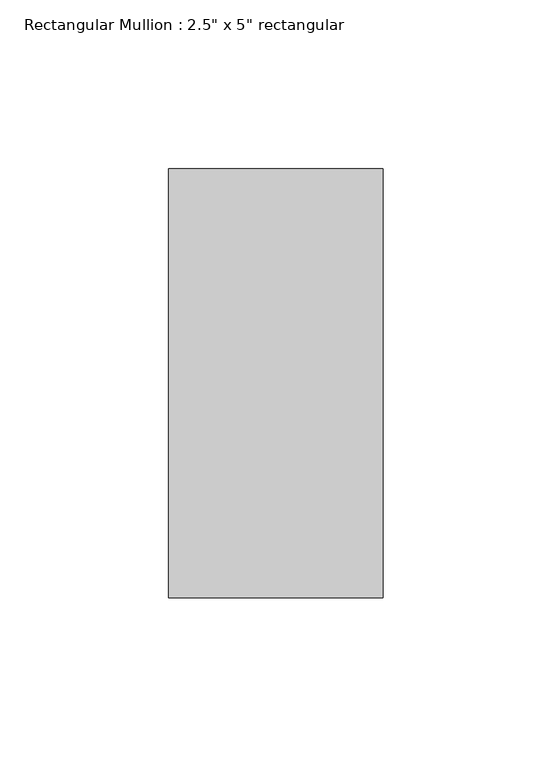
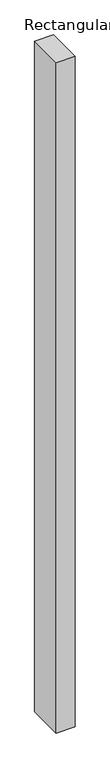
"""IFC4 building model written with IfcOpenShell, lengths in millimetres: member geometry."""

from ifc_helpers import new_model, si_unit, frame, origin, place, context, project, spatial, polyline, outline, extrude, source, transform, mapped, element, save


def member_bd9e6ea3(model_context):
    return source(origin(), model_context, "Body", "SweptSolid", [
        extrude(outline(polyline([(0.0, 63.5), (0.0, -63.5), (-63.5, -63.5), (-63.5, 63.5), (0.0, 63.5)])), frame((0.0, 0.0, -2411.5809615), z_axis=(0.0, 0.0, 1.0), x_axis=(1.0, 0.0, 0.0)), (0.0, 0.0, 1.0), 2411.5809615),
    ])


if __name__ == "__main__":
    model = new_model("IFC4")
    model_context = context("Model", 3, world=origin())
    ifc_project = project(units=[si_unit("LENGTHUNIT", "METRE", prefix="MILLI")], contexts=[model_context])
    site = spatial("IfcSite", under=ifc_project)
    building = spatial("IfcBuilding", under=site)
    placement = place(None, origin())
    member_shape = member_bd9e6ea3(model_context)
    element("IfcMember", 1, ObjectType="Rectangular Mullion : 2.5\" x 5\" rectangular", at=placement, inside=building, context=model_context, shape_type="MappedRepresentation", body=[
        mapped(member_shape, transform((0.0, 0.0, 0.0), x_axis=(1.0, 0.0, 0.0), y_axis=(0.0, 1.0, 0.0), z_axis=(0.0, 0.0, 1.0))),
    ])
    save(model, "model.ifc")

# Revit data of these elements
# Type "Rectangular Mullion : 2.5\" x 5\" rectangular"
#   built-in parameter 1007304 = 0.416667 (stored number, unit not read)
#   built-in parameter 1007301 = 0.104167 (stored number, unit not read)
#   built-in parameter 1007300 = 0.104167 (stored number, unit not read)
# Element 1 (IfcMember, "Rectangular Mullion : 2.5\" x 5\" rectangular")
#   Materials on its faces: "Aluminum"
# Materials
#   "Aluminum": class "Metal", colour RGB 247 247 247, transparency 0, Description = "Aluminum 6061", Cost = 0
